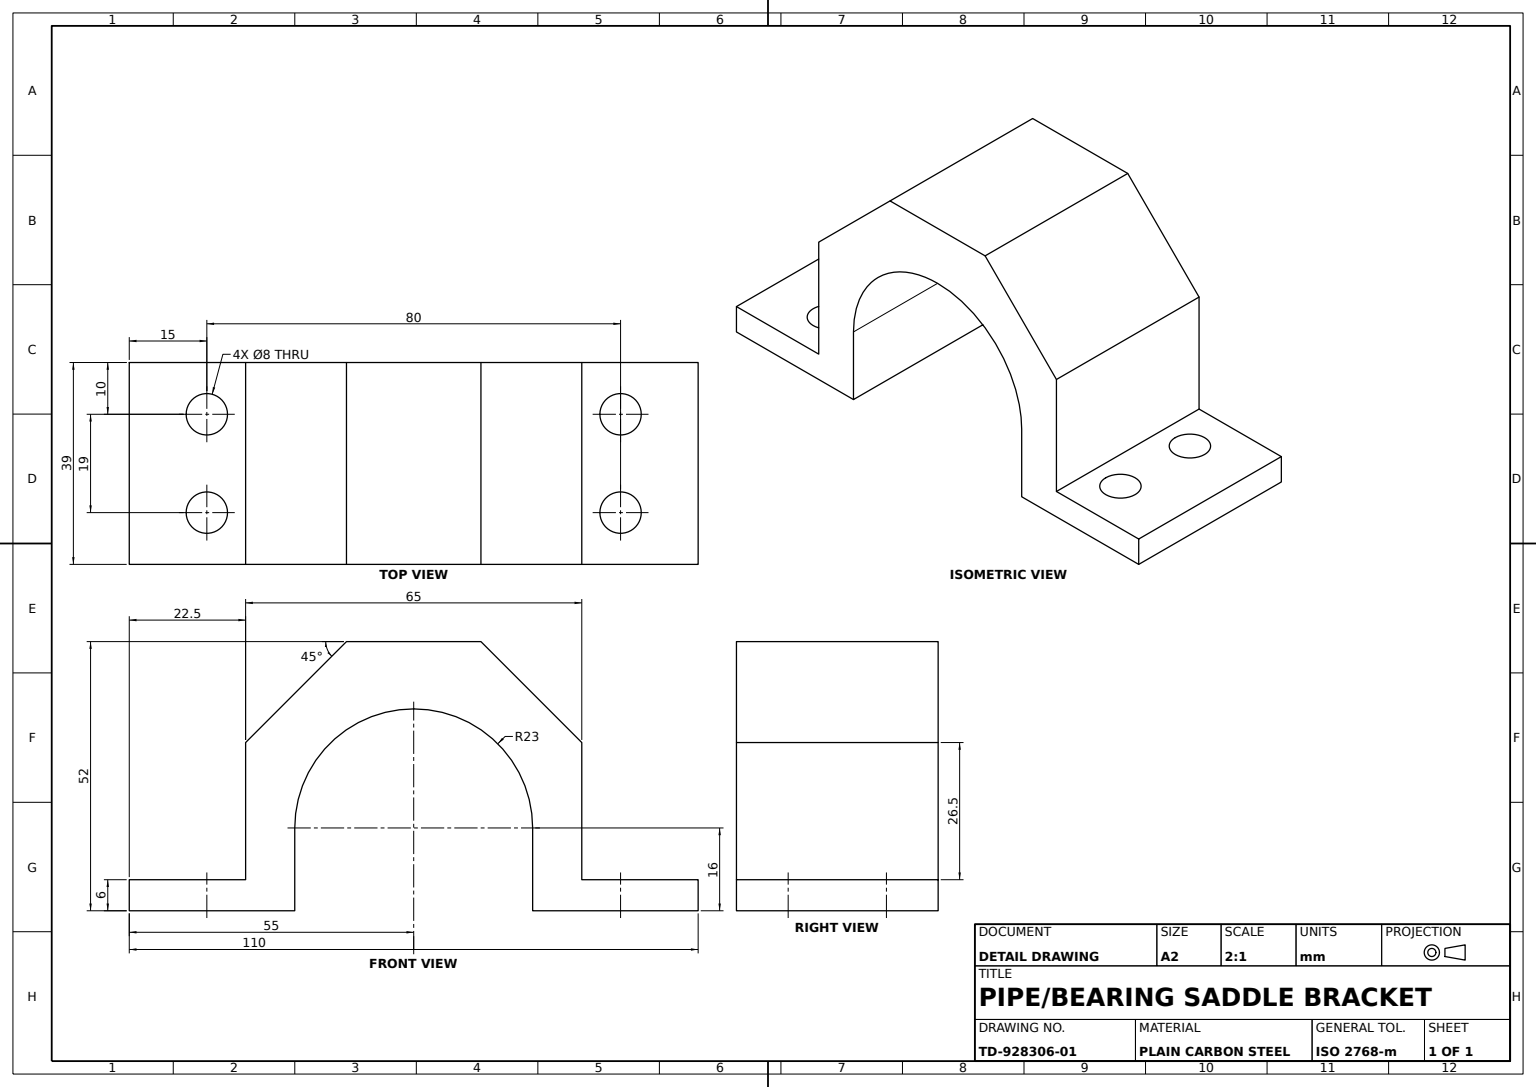
SolidWorks part; units mm, degrees
material "Plain Carbon Steel"
ref_plane "Front Plane" through (0, 0, 0) normal (0, 0, 1) x (1, 0, 0)
ref_plane "Top Plane" through (0, 0, 0) normal (0, 1, 0) x (1, 0, 0)
ref_plane "Right Plane" through (0, 0, 0) normal (1, 0, 0) x (0, 0, -1)
sketch "Base Plate Sketch" plane through (0, 0, 0) normal (0, 0, 1) x (1, 0, 0)
  line L0 (0, 0) -> (110, 0)
  line L1 (110, 0) -> (110, 39)
  line L2 (110, 39) -> (0, 39)
  line L3 (0, 39) -> (0, 0)
  dimension "D1" = 110
  dimension "D2" = 39
extrude "Base Plate 110x39x6" add sketch "Base Plate Sketch" along normal blind 6
sketch "Saddle Body Profile" plane through (0, 0, 0) normal (0, -1, 0) x (1, 0, 0)
  line L0 (55, 6) -> (55, -46)
  line L1 (0, 6) -> (110, 6) construction
  line L2 (42, -46) -> (68, -46)
  line L3 (42, -46) -> (68, -46)
  line L4 (87.5, -26.5) -> (87.5, 0)
  line L5 (0, 0) -> (110, 0) construction
  line L6 (22.5, -26.5) -> (22.5, 0)
  line L7 (42, -46) -> (22.5, -26.5)
  line L8 (68, -46) -> (87.5, -26.5)
  line L9 (55, 6) -> (55, -10)
  line L10 (32, -10) -> (32, 0)
  line L11 (78, -10) -> (78, 0)
  line L12 (22.5, 0) -> (87.5, 0)
  arc A0 (32, -10) -> (78, -10) centre (55, -10) ccw
  point P7 (55, -46)
  point P10 (55, -46)
  line M6 (0, 0) -> (110, 0)
  dimension "D2" = 13
  dimension "D8" = 23
  dimension "D1" = 52
  dimension "D3" = 26.5
  dimension "D4" = 45
  dimension "D5" = 45
  dimension "D6" = 26.5
  dimension "D7" = 16
extrude "Saddle Body 39" add sketch "Saddle Body Profile" against normal blind 39 contours A0 L10 L6 L7 L2 L0 M6 | A0 L0 L2 L8 L4 L11 M6
sketch "Saddle Cutout Sketch" plane through (0, 0, 0) normal (0, -1, 0) x (1, 0, 0)
  line L0 (32, 0) -> (32, 6)
  line L1 (0, 6) -> (110, 6) construction
  line L2 (32, 6) -> (78, 6)
  line L3 (78, 6) -> (78, 0)
  line L4 (78, 0) -> (32, 0)
extrude "Saddle Cutout" cut sketch "Saddle Cutout Sketch" against normal blind 39
sketch "Flange Holes Sketch" plane through (0, 0, 6) normal (0, 0, 1) x (1, 0, 0)
  line L0 (78, 39) -> (32, 39) construction
  line L1 (55, 39) -> (55, 0)
  line L2 (32, 0) -> (78, 0) construction
  line L3 (32, 39) -> (0, 39) construction
  line L4 (0, 0) -> (32, 0) construction
  line L5 (110, 39) -> (78, 39) construction
  line L6 (78, 0) -> (110, 0) construction
  circle A0 centre (15, 29) radius 4
  circle A1 centre (15, 10) radius 4
  circle A2 centre (95, 29) radius 4
  circle A3 centre (95, 10) radius 4
  dimension "D1" = 8
  dimension "D2" = 8
  dimension "D3" = 8
  dimension "D4" = 8
  dimension "D5" = 40
  dimension "D6" = 40
  dimension "D7" = 40
  dimension "D8" = 40
  dimension "D9" = 10
  dimension "D10" = 10
  dimension "D11" = 10
  dimension "D12" = 10
extrude "Flange Holes 4xØ8" cut sketch "Flange Holes Sketch" against normal blind 39 contours A0 | A1 | A2 | A3
